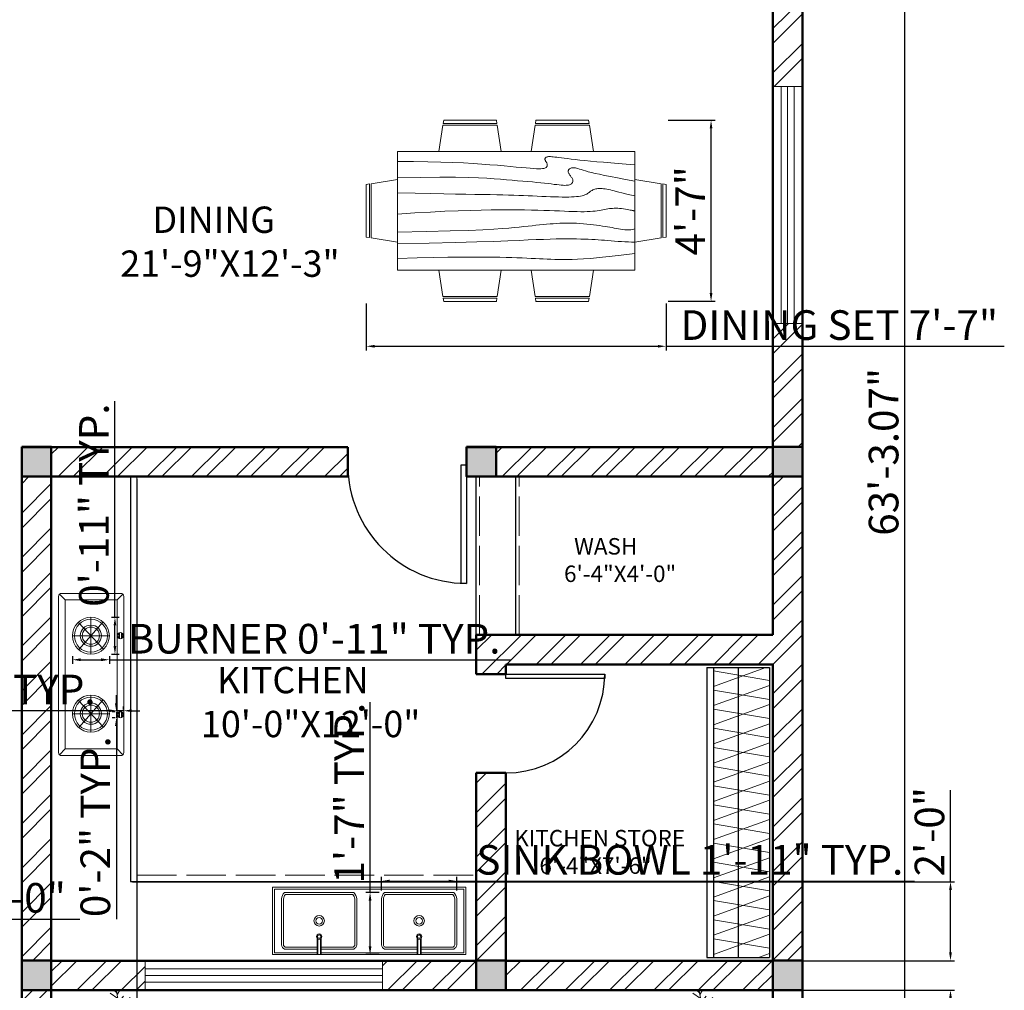
# Model space of a CAD drawing. Units: inches. Extents: x 381 to 1001, y 3003 to 3971.
# Tile 3 of 4: x 702 to 1001, y 3347 to 3641. Entities that reach past the tile are written whole.
import ezdxf

# ---------------------------------------------------------------- set-up
doc = ezdxf.new("R2010")
doc.units = ezdxf.units.IN
doc.linetypes.add('ACAD_ISO02W100', pattern=[15, 12, -3])
for name, color, linetype, lineweight in [('A-ANNO-DIMS', 2, 'Continuous', 18), ('A-AREA-IDEN', 7, 'Continuous', 18), ('A-COLS', 7, 'Continuous', 50), ('A-DOOR', 4, 'Continuous', 25), ('A-EQPM', 8, 'Continuous', 18), ('A-FLOR', 7, 'Continuous', 25), ('A-FLOR-CASE', 8, 'Continuous', 25), ('A-FLOR-CASE-HIDN', 8, 'ACAD_ISO02W100', 13), ('A-FLOR-CASE-PATT', 252, 'Continuous', 13), ('A-FLOR-FIXT', 9, 'Continuous', 18), ('A-FLOR-STRS', 7, 'Continuous', 25), ('A-FLOR-STRS-HIDN', 8, 'ACAD_ISO02W100', 13), ('A-FURN', 8, 'Continuous', 18), ('A-GLAZ', 244, 'Continuous', 18), ('A-WALL', 7, 'Continuous', 50), ('A-WALL-PATT', 252, 'Continuous', 13), ('L-PLNT', 3, 'Continuous', 13)]:
    doc.layers.add(name, color=color, linetype=linetype, lineweight=lineweight)
doc.styles.get("Standard").update_dxf_attribs({"font": 'arial.ttf'})
doc.dimstyles.new('ISO-25', dxfattribs={"dimtxt": 9, "dimasz": 2.5, "dimexe": 1.25, "dimexo": 0.625, "dimtad": 1, "dimlunit": 3, "dimtxsty": 'Standard', "dimcen": 2.5, "dimadec": 0, "dimazin": 0, "dimtfac": 1, "dimtmove": 0, "dimatfit": 3, "dimfxl": 1, "dimarcsym": 0})

# ---------------------------------------------------------------- blocks, each defined once
blk = doc.blocks.new('*U6')
for p, q in [((-40, 0), (-40, 6)), ((0, 0), (0, 6))]:
    blk.add_line(p, q)
blk.add_lwpolyline([(0, 0), (0, -40), (-1.75, -40), (-1.75, 0)], close=True)
blk.add_arc((0, 0), 40, 180, 270)
blk = doc.blocks.new('*U7')
for p, q in [((-40, 0), (-40, 6)), ((0, 0), (0, 6))]:
    blk.add_line(p, q)
blk.add_lwpolyline([(0, 0), (0, -40), (-1.75, -40), (-1.75, 0)], close=True)
blk.add_arc((0, 0), 40, 180, 270)
blk = doc.blocks.new('Dining Set - 36 x 72 in.')
for p, q in [((-22, 27.5), (-22.1562, 26.50042)), ((-22, 27.5), (-6, 27.5)), ((-5.8437, 26.49966), (-6, 27.5)), ((6, 27.5), (5.8438, 26.50042)), ((6, 27.5), (22, 27.5)), ((22.1563, 26.49966), (22, 27.5)), ((-22.2343, 26.00059), (-23.4847, 17.99762)), ((-22.2304, 26), (-5.7608, 26)), ((-5.8416, 26.5), (-22.1534, 26.5)), ((-4.5152, 17.99762), (-5.7655, 25.99926)), ((5.7657, 26.00059), (4.5153, 17.99762)), ((5.7696, 26), (22.2392, 26)), ((22.1584, 26.5), (5.8466, 26.5)), ((23.4848, 17.99762), (22.2345, 25.99926)), ((36, 18), (-36, 18)), ((-36, 18), (-36, -18)), ((36, -18), (36, 18)), ((-44.0006, 8.23428), (-35.9976, 9.48474)), ((44.0006, 8.23428), (35.9976, 9.48474)), ((-45.5, 8), (-44.5004, 8.15617)), ((-45.5, 8), (-45.5, -8)), ((-44.5, -8.15843), (-44.5, 8.15338)), ((-44, 8.23041), (-44, -8.23915)), ((44, 8.23041), (44, -8.23915)), ((44.5, -8.15843), (44.5, 8.15338)), ((45.5, 8), (44.5005, 8.15617)), ((45.5, 8), (45.5, -8)), ((-44.4997, -8.15631), (-45.5, -8)), ((-35.9976, -9.48476), (-43.9993, -8.2345)), ((35.9976, -9.48476), (43.9993, -8.2345)), ((44.4997, -8.15631), (45.5, -8)), ((-36, -18), (36, -18)), ((-22.2343, -26.0006), (-23.4847, -17.99762)), ((-4.5152, -17.99762), (-5.7655, -25.99928)), ((5.7657, -26.0006), (4.5153, -17.99762)), ((23.4848, -17.99762), (22.2345, -25.99928)), ((-22.2304, -26), (-5.7608, -26)), ((-22, -27.5), (-22.1562, -26.50044)), ((-5.8416, -26.5), (-22.1534, -26.5)), ((-5.8437, -26.49967), (-6, -27.5)), ((5.7696, -26), (22.2392, -26)), ((6, -27.5), (5.8438, -26.50044)), ((22.1584, -26.5), (5.8466, -26.5)), ((22.1563, -26.49967), (22, -27.5)), ((-22, -27.5), (-6, -27.5)), ((6, -27.5), (22, -27.5))]:
    blk.add_line(p, q)
for points in [[(-36, 15), (-31.1772, 14.97754), (-26.8079, 14.91406), (-22.8538, 14.81543), (-19.276, 14.6875), (-16.0362, 14.53613), (-13.0957, 14.36718), (-10.4159, 14.18652), (-7.9583, 14), (-5.6904, 13.81315), (-3.6035, 13.63021), (-1.6954, 13.45508), (0.0365, 13.29166), (1.5945, 13.14388), (2.9811, 13.01562), (4.1988, 12.9108), (5.25, 12.83333), (6.1393, 12.78613), (6.8802, 12.76823), (7.4883, 12.77767), (7.9792, 12.8125), (8.3685, 12.87077), (8.6719, 12.95052), (8.9049, 13.0498), (9.0833, 13.16666), (9.2205, 13.29899), (9.3216, 13.44401), (9.3895, 13.59879), (9.4271, 13.76041), (9.4373, 13.92594), (9.4232, 14.09245), (9.3875, 14.257), (9.3333, 14.41666), (9.2638, 14.56917), (9.1836, 14.71484), (9.0975, 14.85465), (9.0104, 14.98958), (8.9272, 15.1206), (8.8529, 15.2487), (8.7922, 15.37483), (8.75, 15.5), (8.7305, 15.62467), (8.7344, 15.74739), (8.7617, 15.86621), (8.8125, 15.97916), (8.8867, 16.08431), (8.9844, 16.17968), (9.1055, 16.26334), (9.25, 16.33333), (9.4189, 16.38802), (9.6172, 16.42708), (9.8506, 16.45052), (10.125, 16.45833), (10.4463, 16.45052), (10.8203, 16.42708), (11.2529, 16.38802), (11.75, 16.33333), (12.3184, 16.26318), (12.9694, 16.17838), (13.7151, 16.07991), (14.5677, 15.96875), (15.5395, 15.84586), (16.6426, 15.71224), (17.8893, 15.56884), (19.2917, 15.41666), (20.859, 15.25667), (22.5879, 15.08984), (24.4721, 14.91715), (26.5052, 14.73958), (28.6809, 14.5581), (30.9929, 14.3737), (33.4347, 14.18733), (36, 14)], [(-36, 10), (-28.9766, 10.14274), (-23.1725, 10.20442), (-18.4241, 10.19775), (-14.5677, 10.13541), (-11.4399, 10.03011), (-8.877, 9.89453), (-6.7154, 9.74137), (-4.7917, 9.58333), (-2.9698, 9.43082), (-1.2246, 9.28515), (0.4415, 9.14534), (2.026, 9.01041), (3.5266, 8.87939), (4.9408, 8.7513), (6.266, 8.62516), (7.5, 8.5), (8.6411, 8.37549), (9.6914, 8.2539), (10.6538, 8.13818), (11.5312, 8.03125), (12.3267, 7.93603), (13.043, 7.85547), (13.6831, 7.79248), (14.25, 7.75), (14.7471, 7.7303), (15.1797, 7.73307), (15.5537, 7.75732), (15.875, 7.80208), (16.1494, 7.86637), (16.3828, 7.94922), (16.5811, 8.04964), (16.75, 8.16666), (16.8944, 8.29915), (17.0143, 8.44531), (17.1089, 8.60319), (17.1771, 8.77083), (17.218, 8.94629), (17.2305, 9.1276), (17.2137, 9.31282), (17.1667, 9.5), (17.0895, 9.6875), (16.987, 9.875), (16.8649, 10.0625), (16.7292, 10.25), (16.5856, 10.4375), (16.4401, 10.625), (16.2985, 10.8125), (16.1667, 11), (16.05, 11.18733), (15.9518, 11.3737), (15.8752, 11.5581), (15.8229, 11.73958), (15.798, 11.91715), (15.8034, 12.08984), (15.842, 12.25667), (15.9167, 12.41666), (16.0295, 12.56836), (16.1784, 12.70833), (16.3605, 12.83268), (16.5729, 12.9375), (16.8127, 13.01888), (17.0768, 13.07291), (17.3625, 13.0957), (17.6667, 13.08333), (17.9894, 13.03312), (18.3418, 12.94726), (18.7382, 12.82918), (19.1927, 12.68229), (19.7195, 12.51001), (20.3327, 12.31575), (21.0465, 12.10294), (21.875, 11.875), (22.8357, 11.63354), (23.959, 11.37304), (25.2786, 11.08618), (26.8282, 10.76562), (28.6414, 10.40405), (30.752, 9.99414), (33.1936, 9.52856), (36, 9)], [(-36, 5.5), (-30.7157, 5.3348), (-26.069, 5.20963), (-21.9946, 5.11767), (-18.4271, 5.05208), (-15.3009, 5.00602), (-12.5508, 4.97265), (-10.1112, 4.94515), (-7.9167, 4.91666), (-5.909, 4.88167), (-4.0586, 4.83984), (-2.3429, 4.79215), (-0.7396, 4.73958), (0.7739, 4.6831), (2.22, 4.6237), (3.6213, 4.56233), (5, 4.5), (6.373, 4.43782), (7.7344, 4.3776), (9.0723, 4.32129), (10.375, 4.27083), (11.6309, 4.22819), (12.8281, 4.19531), (13.9551, 4.17415), (15, 4.16666), (15.954, 4.17448), (16.819, 4.19791), (17.6001, 4.23698), (18.3021, 4.29166), (18.9299, 4.36198), (19.4883, 4.44791), (19.9823, 4.54948), (20.4167, 4.66666), (20.7969, 4.79899), (21.1302, 4.94401), (21.4245, 5.09879), (21.6875, 5.26041), (21.9271, 5.42594), (22.1511, 5.59245), (22.3672, 5.757), (22.5834, 5.91666), (22.8065, 6.06868), (23.0404, 6.21093), (23.2879, 6.34147), (23.5521, 6.45833), (23.8358, 6.55957), (24.142, 6.64323), (24.4735, 6.70735), (24.8334, 6.75), (25.2235, 6.76969), (25.642, 6.76692), (26.0858, 6.74267), (26.5521, 6.69791), (27.0379, 6.63362), (27.5404, 6.55078), (28.0565, 6.45036), (28.5834, 6.33333), (29.1242, 6.19987), (29.7071, 6.04687), (30.3661, 5.87044), (31.1354, 5.66666), (32.0493, 5.43164), (33.142, 5.16146), (34.4475, 4.85221), (36, 4.5)], [(-36, -1), (-30.7915, -0.6591), (-26.0195, -0.38216), (-21.6519, -0.16284), (-17.6563, 0.00521), (-14.0005, 0.12833), (-10.6523, 0.21289), (-7.5796, 0.26522), (-4.75, 0.29166), (-2.134, 0.29793), (0.2878, 0.28711), (2.5317, 0.26163), (4.6146, 0.22396), (6.5529, 0.17651), (8.3633, 0.12174), (10.0623, 0.06209), (11.6667, 0), (13.1899, -0.06201), (14.6341, -0.1211), (15.9982, -0.17432), (17.2813, -0.21875), (18.4823, -0.25147), (19.6003, -0.26953), (20.6343, -0.27002), (21.5834, -0.25), (22.4481, -0.20768), (23.2357, -0.14584), (23.9549, -0.06836), (24.6146, 0.02083), (25.2235, 0.11784), (25.7904, 0.21875), (26.3241, 0.31966), (26.8334, 0.41666), (27.3265, 0.50618), (27.8099, 0.58593), (28.2894, 0.65397), (28.7709, 0.70833), (29.2601, 0.74707), (29.763, 0.76823), (30.2855, 0.76985), (30.8334, 0.75), (31.4088, 0.70784), (31.9994, 0.64713), (32.589, 0.57275), (33.1615, 0.48958), (33.7008, 0.4025), (34.1908, 0.3164), (34.6153, 0.23616), (34.9584, 0.16666), (35.2099, 0.11165), (35.3848, 0.07031), (35.504, 0.04069), (35.5886, 0.02083), (35.6594, 0.00879), (35.7377, 0.0026), (35.8442, 0.00032), (36, 0)], [(-36, -6.5), (-27.1843, -6.31267), (-20.084, -6.1263), (-14.469, -5.9419), (-10.1094, -5.76042), (-6.7752, -5.58285), (-4.2363, -5.41016), (-2.2629, -5.24333), (-0.625, -5.08334), (0.8708, -4.93099), (2.2715, -4.78646), (3.5872, -4.64974), (4.8281, -4.52084), (6.0046, -4.39974), (7.127, -4.28646), (8.2053, -4.18099), (9.25, -4.08334), (10.2705, -3.99382), (11.2734, -3.91407), (12.2647, -3.84603), (13.25, -3.79167), (14.2354, -3.75293), (15.2266, -3.73177), (16.2295, -3.73015), (17.25, -3.75), (18.2912, -3.79248), (19.3451, -3.85547), (20.4009, -3.93604), (21.4479, -4.03125), (22.4754, -4.13819), (23.4727, -4.25391), (24.4289, -4.37549), (25.3334, -4.5), (26.1785, -4.62492), (26.9694, -4.74935), (27.7145, -4.87281), (28.4219, -4.99479), (29.1, -5.11483), (29.7572, -5.23242), (30.4016, -5.34709), (31.0417, -5.45834), (31.6837, -5.56437), (32.3262, -5.65821), (32.9658, -5.73153), (33.599, -5.77604), (34.2224, -5.78345), (34.8327, -5.74545), (35.4264, -5.65373), (36, -5.5)], [(-36, -10), (-26.4022, -9.81299), (-18.4675, -9.62891), (-11.9839, -9.45069), (-6.7396, -9.28125), (-2.5226, -9.12354), (0.8789, -8.98047), (3.6769, -8.85498), (6.0833, -8.75), (8.2767, -8.66765), (10.3021, -8.60677), (12.1712, -8.56543), (13.8958, -8.54167), (15.4876, -8.53353), (16.9583, -8.53907), (18.3197, -8.55632), (19.5834, -8.58334), (20.7616, -8.61841), (21.8685, -8.66081), (22.9188, -8.71004), (23.9271, -8.76563), (24.9081, -8.82707), (25.8763, -8.89388), (26.8465, -8.96558), (27.8334, -9.04167), (28.8474, -9.12118), (29.8828, -9.20117), (30.93, -9.27824), (31.9792, -9.34896), (33.0205, -9.40991), (34.0443, -9.45768), (35.0407, -9.48885), (36, -9.5)], [(-36, -14.5), (-30.0881, -14.33513), (-25.0332, -14.21224), (-20.7312, -14.12647), (-17.0781, -14.07292), (-13.97, -14.04671), (-11.3027, -14.04297), (-8.9724, -14.05681), (-6.875, -14.08334), (-4.9224, -14.11833), (-3.0905, -14.16016), (-1.3709, -14.20785), (0.2448, -14.26042), (1.7647, -14.3169), (3.1973, -14.3763), (4.5507, -14.43767), (5.8333, -14.5), (7.0554, -14.5621), (8.235, -14.62175), (9.3922, -14.67652), (10.5469, -14.72396), (11.7192, -14.76164), (12.929, -14.78711), (14.1965, -14.79794), (15.5417, -14.79167), (16.9933, -14.76424), (18.6152, -14.70508), (20.4804, -14.60197), (22.6615, -14.44271), (25.2312, -14.21509), (28.2624, -13.9069), (31.8277, -13.50594), (36, -13)]]:
    blk.add_lwpolyline(points)
blk = doc.blocks.new('*U15')
for p, q in [((-10.186, 53.64), (-13.084, 55.962)), ((0, 0), (-10.5, 57)), ((-9.099, 51.782), (-6.563, 55.962)), ((-7.288, 39.707), (-21.778, 46.673)), ((-8.737, 47.138), (-17.069, 52.711)), ((-7.65, 43.423), (-2.578, 49.46)), ((-5.839, 35.992), (4.667, 48.067)), ((-5.114, 27.632), (10.463, 46.673)), ((-3.665, 19.273), (-27.574, 35.527)), ((-5.114, 28.097), (-24.676, 40.636)), ((-2.941, 16.486), (8.652, 37.85)), ((22.055, 7.198), (27.489, 32.277)), ((27, 9), (48, 36)), ((27.127, 9.056), (31.112, 35.992)), ((35.096, 32.741), (37.27, 22.524)), ((38.719, 34.134), (41.979, 28.561)), ((44.153, 36.456), (45.239, 32.741)), ((-31.5, 4.5), (-52.5, 25.5)), ((-48.585, 21.131), (-49.309, 29.026)), ((-43.513, 28.561), (-42.427, 15.558)), ((-38.442, 26.239), (-34.819, 7.663)), ((-35.544, 28.097), (-24.314, 3.947)), ((-14.533, 2.09), (-30.834, 25.31)), ((-24.314, 23.917), (-2.941, 13.7)), ((-1.129, 6.734), (9.014, 26.704)), ((3.942, 1.625), (11.187, 24.381)), ((10.101, 3.483), (17.708, 26.239)), ((16.259, 5.805), (23.142, 31.348)), ((31.836, 30.883), (32.561, 16.486)), ((40.53, 25.775), (48.862, 24.846)), ((43.791, 29.954), (51.036, 30.883)), ((-47.498, 19.737), (-55.83, 18.344)), ((-40.615, 13.7), (-55.105, 10.913)), ((-20.691, 13.7), (-1.129, 4.876)), ((29.662, 12.307), (48.137, 6.269)), ((33.285, 16.486), (48.862, 10.913)), ((36.183, 19.737), (48.137, 17.88)), ((-33.37, 6.269), (-52.207, 5.34)), ((-28.299, 3.483), (-47.86, -5.805)), ((-21.416, 3.018), (-38.079, -8.128)), ((0, 0), (-31.5, 4.5)), ((-15.982, 2.09), (-30.11, -9.521)), ((0, 0), (-22.5, -19.5)), ((-6.563, 1.161), (-21.416, -8.128)), ((0, 0), (27, 9)), ((0, 0), (18, -22.5)), ((6.478, 1.625), (26.04, -8.592)), ((11.187, 3.483), (30.749, -5.805)), ((18.07, 5.805), (35.096, -3.483)), ((24.229, 7.663), (46.688, 1.625)), ((-6.563, -5.805), (-19.967, -9.985)), ((-9.461, -8.592), (-6.201, -23.453)), ((-4.752, -3.483), (-3.665, -14.629)), ((2.493, -3.019), (-1.491, -20.202)), ((1.769, -2.555), (24.229, -9.521)), ((5.029, -6.27), (2.131, -25.775)), ((7.565, -9.056), (32.198, -14.629)), ((-17.431, -15.094), (-42.789, -18.809)), ((-22.5, -19.5), (-37.5, -45)), ((-15.257, -12.772), (-30.11, -12.772)), ((-20.691, -18.345), (-17.793, -44.352)), ((-17.069, -15.094), (-12.721, -40.172)), ((-13.446, -11.378), (-8.737, -32.741)), ((9.014, -11.378), (3.58, -35.992)), ((14.085, -16.951), (6.478, -40.172)), ((12.274, -15.094), (36.907, -18.809)), ((16.259, -19.738), (36.183, -22.989)), ((-28.299, -29.026), (-42.789, -31.348)), ((-24.314, -21.596), (-42.427, -22.06)), ((-26.849, -26.24), (-40.253, -25.775)), ((-29.023, -30.884), (-27.936, -43.887)), ((-25.038, -23.918), (-22.865, -45.281)), ((18.07, -22.524), (8.289, -45.745)), ((20.244, -30.419), (15.897, -44.816)), ((18, -22.5), (27, -52.5)), ((18.433, -22.524), (40.53, -29.026)), ((19.157, -25.311), (38.719, -33.206)), ((-30.834, -34.135), (-42.427, -35.528)), ((-34.457, -39.708), (-40.978, -42.494)), ((-32.646, -36.921), (-31.921, -44.352)), ((22.78, -37.85), (19.519, -48.532)), ((21.331, -32.741), (39.081, -40.636)), ((22.78, -38.314), (34.372, -44.816)), ((24.591, -45.745), (23.142, -50.854)), ((24.591, -43.423), (30.749, -47.603)), ((26.764, -49.925), (28.213, -50.854))]:
    blk.add_line(p, q)
blk = doc.blocks.new('*D22')
at = {"layer": 'A-ANNO-DIMS', "color": 0, "lineweight": -2, "transparency": 16777216}
for p, q in [((940.7, 3889.64), (972.35, 3889.64)), ((971.1, 3887.14), (971.1, 3133.06)), ((940.7, 3130.56), (972.35, 3130.56))]:
    blk.add_line(p, q, dxfattribs=at)
at = {"layer": 'A-ANNO-DIMS', "color": 0, "transparency": 16777216}
for points in [[(970.69, 3887.14), (971.52, 3887.14), (971.1, 3889.64)], [(970.69, 3133.06), (971.52, 3133.06), (971.1, 3130.56)]]:
    blk.add_solid(points, dxfattribs=at)
at = {"layer": 'Defpoints', "color": 0, "transparency": 16777216}
for p in [(940.08, 3889.64), (940.08, 3130.56), (971.1, 3130.56)]:
    blk.add_point(p, dxfattribs=at)
at = {"layer": 'A-ANNO-DIMS', "color": 0, "transparency": 16777216, "insert": (965.88, 3510.1), "char_height": 9, "attachment_point": 5, "rotation": 90}
blk.add_mtext('63\'-3.07"', dxfattribs=at)
blk = doc.blocks.new('WIN-72X9')
for p, q in [((72, 6.5), (0, 6.5)), ((72, 4.5), (0, 4.5)), ((72, 2.5), (0, 2.5))]:
    blk.add_line(p, q)
blk.add_lwpolyline([(72, 9), (72, 0), (0, 0), (0, 9)], close=True)
blk = doc.blocks.new('COLUMN-9X9')
h = blk.add_hatch(color=256)
h.dxf.hatch_style = 1
h.paths.add_polyline_path([(9, 9), (0, 9), (0, 0), (9, 0)])
blk.add_lwpolyline([(0, 9), (9, 9), (9, 0), (0, 0)], close=True)
blk = doc.blocks.new('SINK-BOWL-WITH-TAP')
for p, q in [((10.86, 4.95), (10.86, 0)), ((11.06, 4.79), (11.06, 0)), ((11.86, 4.79), (11.86, 0)), ((12.06, 4.95), (12.06, 0))]:
    blk.add_line(p, q)
for points in [[(12.06, 1.68), (22.01, 1.68, 0.204191), (22.91, 2.94), (22.91, 16.97, 0.131614), (22.01, 18.91), (0.9, 18.91, 0.131614), (0, 16.97), (0, 2.94, 0.204191), (0.9, 1.68), (10.86, 1.68)], [(12.06, 2.28), (21.83, 2.28, 0.163903), (22.31, 3.01), (22.31, 16.91, 0.108554), (21.72, 18.31), (1.19, 18.31, 0.108554), (0.6, 16.91), (0.6, 3.01, 0.163903), (1.09, 2.28), (10.86, 2.28)]]:
    blk.add_lwpolyline(points, format="xyb")
for centre, radius in [((11.46, 10.29), 1.59), ((11.46, 10.29), 0.993), ((11.46, 5.49), 0.805), ((11.46, 5.49), 0.505)]:
    blk.add_circle(centre, radius)
blk = doc.blocks.new('COOKTOP-BURNER')
for p, q in [((9.48, 1.55), (1.74, 9.68)), ((1.93, 1.38), (9.3, 9.85)), ((5.61, 11.23), (5.61, 0)), ((0, 5.61), (11.23, 5.61))]:
    blk.add_line(p, q)
for radius in [5.61, 5.01, 3.21, 2.61]:
    blk.add_circle((5.61, 5.61), radius)
blk = doc.blocks.new('COOKTOP-KNOB')
for p, q in [((0.64, 1.83), (0.64, 0.05)), ((1.24, 1.83), (1.24, 0.05))]:
    blk.add_line(p, q)
blk.add_circle((0.94, 0.94), 0.94)
for start, end in [(117.9584, 242.0416), (297.9584, 62.0416)]:
    blk.add_arc((0.94, 0.94), 0.64, start, end)
blk = doc.blocks.new('*D42')
at = {"layer": 'A-ANNO-DIMS', "color": 0, "lineweight": -2, "transparency": 16777216}
for p, q in [((812.27, 3376.93), (812.27, 3380.99)), ((835.18, 3376.93), (835.18, 3380.99)), ((814.77, 3379.74), (832.68, 3379.74)), ((835.18, 3379.74), (974.09, 3379.74))]:
    blk.add_line(p, q, dxfattribs=at)
at = {"layer": 'A-ANNO-DIMS', "color": 0, "transparency": 16777216}
for points in [[(814.77, 3380.16), (814.77, 3379.33), (812.27, 3379.74)], [(832.68, 3380.16), (832.68, 3379.33), (835.18, 3379.74)]]:
    blk.add_solid(points, dxfattribs=at)
at = {"layer": 'Defpoints', "color": 0, "transparency": 16777216}
for p in [(835.18, 3379.74), (812.27, 3376.31), (835.18, 3376.31)]:
    blk.add_point(p, dxfattribs=at)
at = {"layer": 'A-ANNO-DIMS', "color": 0, "transparency": 16777216, "insert": (905.89, 3385.03), "char_height": 9, "attachment_point": 5}
blk.add_mtext('SINK BOWL 1\'-11" TYP.', dxfattribs=at)
blk = doc.blocks.new('*D43')
at = {"layer": 'A-ANNO-DIMS', "color": 0, "lineweight": -2, "transparency": 16777216}
for p, q in [((808.83, 3376.31), (808.83, 3434.07)), ((811.64, 3376.31), (807.58, 3376.31)), ((808.83, 3359.9), (808.83, 3373.81)), ((811.64, 3357.4), (807.58, 3357.4))]:
    blk.add_line(p, q, dxfattribs=at)
at = {"layer": 'A-ANNO-DIMS', "color": 0, "transparency": 16777216}
for points in [[(808.41, 3373.81), (809.24, 3373.81), (808.83, 3376.31)], [(808.41, 3359.9), (809.24, 3359.9), (808.83, 3357.4)]]:
    blk.add_solid(points, dxfattribs=at)
at = {"layer": 'Defpoints', "color": 0, "transparency": 16777216}
for p in [(808.83, 3376.31), (812.27, 3376.31), (812.27, 3357.4)]:
    blk.add_point(p, dxfattribs=at)
at = {"layer": 'A-ANNO-DIMS', "color": 0, "transparency": 16777216, "insert": (803.68, 3406.44), "char_height": 9, "attachment_point": 5, "rotation": 90}
blk.add_mtext('1\'-7" TYP.', dxfattribs=at)
blk = doc.blocks.new('*D44')
at = {"layer": 'A-ANNO-DIMS', "color": 0, "lineweight": -2, "transparency": 16777216}
for p, q in [((718.48, 3448.02), (718.48, 3445.71)), ((720.98, 3446.96), (727.2, 3446.96)), ((729.7, 3448.02), (729.7, 3445.71)), ((729.7, 3446.96), (851.49, 3446.96))]:
    blk.add_line(p, q, dxfattribs=at)
at = {"layer": 'A-ANNO-DIMS', "color": 0, "transparency": 16777216}
for points in [[(720.98, 3447.38), (720.98, 3446.54), (718.48, 3446.96)], [(727.2, 3447.38), (727.2, 3446.54), (729.7, 3446.96)]]:
    blk.add_solid(points, dxfattribs=at)
at = {"layer": 'Defpoints', "color": 0, "transparency": 16777216}
for p in [(718.48, 3448.64), (729.7, 3448.64), (729.7, 3446.96)]:
    blk.add_point(p, dxfattribs=at)
at = {"layer": 'A-ANNO-DIMS', "color": 0, "transparency": 16777216, "insert": (791.85, 3452.18), "char_height": 9, "attachment_point": 5}
blk.add_mtext('BURNER 0\'-11" TYP.', dxfattribs=at)
blk = doc.blocks.new('*D45')
at = {"layer": 'A-ANNO-DIMS', "color": 0, "lineweight": -2, "transparency": 16777216}
for p, q in [((731.39, 3459.87), (731.39, 3525.47)), ((730.33, 3459.87), (732.64, 3459.87)), ((731.39, 3451.14), (731.39, 3457.37)), ((730.33, 3448.64), (732.64, 3448.64))]:
    blk.add_line(p, q, dxfattribs=at)
at = {"layer": 'A-ANNO-DIMS', "color": 0, "transparency": 16777216}
for points in [[(730.97, 3457.37), (731.8, 3457.37), (731.39, 3459.87)], [(730.97, 3451.14), (731.8, 3451.14), (731.39, 3448.64)]]:
    blk.add_solid(points, dxfattribs=at)
at = {"layer": 'Defpoints', "color": 0, "transparency": 16777216}
for p in [(729.7, 3459.87), (731.39, 3459.87), (729.7, 3448.64)]:
    blk.add_point(p, dxfattribs=at)
at = {"layer": 'A-ANNO-DIMS', "color": 0, "transparency": 16777216, "insert": (726.17, 3493.92), "char_height": 9, "attachment_point": 5, "rotation": 90}
blk.add_mtext('0\'-11" TYP.', dxfattribs=at)
blk = doc.blocks.new('*D46')
at = {"layer": 'A-ANNO-DIMS', "color": 0, "lineweight": -2, "transparency": 16777216}
for p, q in [((729.6, 3431.47), (632.26, 3431.47)), ((732.1, 3431.81), (732.1, 3432.72)), ((733.98, 3431.47), (732.1, 3431.47)), ((733.98, 3431.81), (733.98, 3432.72)), ((736.48, 3431.47), (738.98, 3431.47))]:
    blk.add_line(p, q, dxfattribs=at)
at = {"layer": 'A-ANNO-DIMS', "color": 0, "transparency": 16777216}
for points in [[(729.6, 3431.88), (729.6, 3431.05), (732.1, 3431.47)], [(736.48, 3431.88), (736.48, 3431.05), (733.98, 3431.47)]]:
    blk.add_solid(points, dxfattribs=at)
at = {"layer": 'Defpoints', "color": 0, "transparency": 16777216}
for p in [(732.1, 3431.47), (732.1, 3431.18), (733.98, 3431.18)]:
    blk.add_point(p, dxfattribs=at)
at = {"layer": 'A-ANNO-DIMS', "color": 0, "transparency": 16777216, "insert": (679.68, 3436.75), "char_height": 9, "attachment_point": 5}
blk.add_mtext('KNOB 0\'-2" TYP.', dxfattribs=at)
blk = doc.blocks.new('*D47')
at = {"layer": 'A-ANNO-DIMS', "color": 0, "lineweight": -2, "transparency": 16777216}
for p, q in [((731.82, 3433.68), (731.82, 3436.18)), ((731.47, 3431.18), (730.57, 3431.18)), ((731.82, 3431.18), (731.82, 3429.3)), ((731.47, 3429.3), (730.57, 3429.3)), ((731.82, 3426.8), (731.82, 3368.19))]:
    blk.add_line(p, q, dxfattribs=at)
at = {"layer": 'A-ANNO-DIMS', "color": 0, "transparency": 16777216}
for points in [[(731.4, 3433.68), (732.23, 3433.68), (731.82, 3431.18)], [(731.4, 3426.8), (732.23, 3426.8), (731.82, 3429.3)]]:
    blk.add_solid(points, dxfattribs=at)
at = {"layer": 'Defpoints', "color": 0, "transparency": 16777216}
for p in [(732.1, 3431.18), (731.82, 3429.3), (732.1, 3429.3)]:
    blk.add_point(p, dxfattribs=at)
at = {"layer": 'A-ANNO-DIMS', "color": 0, "transparency": 16777216, "insert": (726.6, 3396.25), "char_height": 9, "attachment_point": 5, "rotation": 90}
blk.add_mtext('0\'-2" TYP.', dxfattribs=at)
blk = doc.blocks.new('*D48')
at = {"layer": 'A-ANNO-DIMS', "color": 0, "lineweight": -2, "transparency": 16777216}
for p, q in [((807.69, 3555.18), (807.69, 3540.91)), ((898.69, 3555.18), (898.69, 3540.91)), ((810.19, 3542.16), (896.19, 3542.16)), ((898.69, 3542.16), (1001.36, 3542.16))]:
    blk.add_line(p, q, dxfattribs=at)
at = {"layer": 'A-ANNO-DIMS', "color": 0, "transparency": 16777216}
for points in [[(810.19, 3542.57), (810.19, 3541.74), (807.69, 3542.16)], [(896.19, 3542.57), (896.19, 3541.74), (898.69, 3542.16)]]:
    blk.add_solid(points, dxfattribs=at)
at = {"layer": 'Defpoints', "color": 0, "transparency": 16777216}
for p in [(807.69, 3555.81), (898.69, 3555.81), (898.69, 3542.16)]:
    blk.add_point(p, dxfattribs=at)
at = {"layer": 'A-ANNO-DIMS', "color": 0, "transparency": 16777216, "insert": (951.27, 3547.43), "char_height": 9, "attachment_point": 5}
blk.add_mtext('DINING SET 7\'-7"', dxfattribs=at)
blk = doc.blocks.new('*D49')
at = {"layer": 'A-ANNO-DIMS', "color": 0, "lineweight": -2, "transparency": 16777216}
for p, q in [((899.31, 3610.81), (913.59, 3610.81)), ((912.34, 3558.31), (912.34, 3608.31)), ((899.31, 3555.81), (913.59, 3555.81))]:
    blk.add_line(p, q, dxfattribs=at)
at = {"layer": 'A-ANNO-DIMS', "color": 0, "transparency": 16777216}
for points in [[(911.92, 3608.31), (912.75, 3608.31), (912.34, 3610.81)], [(911.92, 3558.31), (912.75, 3558.31), (912.34, 3555.81)]]:
    blk.add_solid(points, dxfattribs=at)
at = {"layer": 'Defpoints', "color": 0, "transparency": 16777216}
for p in [(898.69, 3610.81), (912.34, 3610.81), (898.69, 3555.81)]:
    blk.add_point(p, dxfattribs=at)
at = {"layer": 'A-ANNO-DIMS', "color": 0, "transparency": 16777216, "insert": (907.21, 3583.31), "char_height": 9, "attachment_point": 5, "rotation": 90}
blk.add_mtext('4\'-7"', dxfattribs=at)
blk = doc.blocks.new('*D50')
at = {"layer": 'A-ANNO-DIMS', "color": 0, "lineweight": -2, "transparency": 16777216}
for p, q in [((535.37, 3376.58), (535.37, 3366.95)), ((595.37, 3376.58), (595.37, 3366.95)), ((537.87, 3368.2), (592.87, 3368.2)), ((595.37, 3368.2), (720.75, 3368.2))]:
    blk.add_line(p, q, dxfattribs=at)
at = {"layer": 'A-ANNO-DIMS', "color": 0, "transparency": 16777216}
for points in [[(537.87, 3368.62), (537.87, 3367.79), (535.37, 3368.2)], [(592.87, 3368.62), (592.87, 3367.79), (595.37, 3368.2)]]:
    blk.add_solid(points, dxfattribs=at)
at = {"layer": 'Defpoints', "color": 0, "transparency": 16777216}
for p in [(535.37, 3377.2), (595.37, 3377.2), (595.37, 3368.2)]:
    blk.add_point(p, dxfattribs=at)
at = {"layer": 'A-ANNO-DIMS', "color": 0, "transparency": 16777216, "insert": (659.31, 3373.48), "char_height": 9, "attachment_point": 5}
blk.add_mtext('COFFEE TABLE 5\'-0"', dxfattribs=at)
blk = doc.blocks.new('*D57')
at = {"layer": 'A-ANNO-DIMS', "color": 0, "lineweight": -2, "transparency": 16777216}
for p, q in [((703.7, 3346.64), (986.28, 3346.64)), ((985.03, 3298.06), (985.03, 3344.14)), ((703.7, 3295.56), (986.28, 3295.56))]:
    blk.add_line(p, q, dxfattribs=at)
at = {"layer": 'A-ANNO-DIMS', "color": 0, "transparency": 16777216}
for points in [[(984.61, 3344.14), (985.44, 3344.14), (985.03, 3346.64)], [(984.61, 3298.06), (985.44, 3298.06), (985.03, 3295.56)]]:
    blk.add_solid(points, dxfattribs=at)
at = {"layer": 'Defpoints', "color": 0, "transparency": 16777216}
for p in [(703.08, 3346.64), (985.03, 3346.64), (703.08, 3295.56)]:
    blk.add_point(p, dxfattribs=at)
at = {"layer": 'A-ANNO-DIMS', "color": 0, "transparency": 16777216, "insert": (979.81, 3321.1), "char_height": 9, "attachment_point": 5, "rotation": 90}
blk.add_mtext('4\'-3"', dxfattribs=at)
blk = doc.blocks.new('*D59')
at = {"layer": 'A-ANNO-DIMS', "color": 0, "lineweight": -2, "transparency": 16777216}
for p, q in [((712.08, 3502.01), (712.08, 3002.98)), ((738.08, 3501.94), (738.08, 3002.98)), ((714.58, 3004.23), (735.58, 3004.23))]:
    blk.add_line(p, q, dxfattribs=at)
at = {"layer": 'A-ANNO-DIMS', "color": 0, "transparency": 16777216}
for points in [[(714.58, 3004.64), (714.58, 3003.81), (712.08, 3004.23)], [(735.58, 3004.64), (735.58, 3003.81), (738.08, 3004.23)]]:
    blk.add_solid(points, dxfattribs=at)
at = {"layer": 'Defpoints', "color": 0, "transparency": 16777216}
for p in [(712.08, 3502.64), (738.08, 3502.56), (738.08, 3004.23)]:
    blk.add_point(p, dxfattribs=at)
at = {"layer": 'A-ANNO-DIMS', "color": 0, "transparency": 16777216, "insert": (725.08, 3009.37), "char_height": 9, "attachment_point": 5}
blk.add_mtext('2\'-2"', dxfattribs=at)
blk = doc.blocks.new('*D60')
at = {"layer": 'A-ANNO-DIMS', "color": 0, "lineweight": -2, "transparency": 16777216}
for p, q in [((985.03, 3379.56), (985.03, 3407.39)), ((736.7, 3379.56), (986.28, 3379.56)), ((985.03, 3358.06), (985.03, 3377.06)), ((712.7, 3355.56), (986.28, 3355.56))]:
    blk.add_line(p, q, dxfattribs=at)
at = {"layer": 'A-ANNO-DIMS', "color": 0, "transparency": 16777216}
for points in [[(984.61, 3377.06), (985.44, 3377.06), (985.03, 3379.56)], [(984.61, 3358.06), (985.44, 3358.06), (985.03, 3355.56)]]:
    blk.add_solid(points, dxfattribs=at)
at = {"layer": 'Defpoints', "color": 0, "transparency": 16777216}
for p in [(736.08, 3379.56), (985.03, 3379.56), (712.08, 3355.56)]:
    blk.add_point(p, dxfattribs=at)
at = {"layer": 'A-ANNO-DIMS', "color": 0, "transparency": 16777216, "insert": (979.81, 3394.73), "char_height": 9, "attachment_point": 5, "rotation": 90}
blk.add_mtext('2\'-0"', dxfattribs=at)

msp = doc.modelspace()

# ---------------------------------------------------------------- hatches: boundary and pattern name
at = {"layer": 'A-FLOR-CASE-PATT'}
h = msp.add_hatch(dxfattribs=at)
h.set_pattern_fill('ANSI31', color=256, scale=1.72204, angle=-25.1679, style=0)
h.paths.add_polyline_path([(913.078, 3356.565), (930.078, 3356.565), (930.078, 3444.565), (913.078, 3444.565)])
h = msp.add_hatch(dxfattribs=at)
h.set_pattern_fill('ANSI31', color=256, scale=1.80506, angle=125.416, style=0)
h.paths.add_polyline_path([(913.078, 3356.565), (930.078, 3356.565), (930.078, 3444.565), (913.078, 3444.565)])
at = {"layer": 'A-WALL-PATT'}
h = msp.add_hatch(dxfattribs=at)
h.set_pattern_fill('ANSI32', color=256)
h.paths.add_polyline_path([(652.078, 3667.565), (487.078, 3667.565), (487.078, 3658.565), (631.078, 3658.565), (631.078, 3655.565), (634.678, 3655.565), (640.078, 3655.565), (640.078, 3658.565), (652.078, 3658.565)])
h.paths.add_polyline_path([(487.078, 3658.637), (478.078, 3658.637), (478.078, 3634.565), (487.078, 3634.565)])
h.paths.add_polyline_path([(487.078, 3703.565), (478.078, 3703.565), (478.078, 3667.637), (487.078, 3667.637)])
h.paths.add_polyline_path([(661.078, 3811.637), (652.078, 3811.637), (652.078, 3706.565), (661.078, 3706.565)])
h.paths.add_polyline_path([(661.078, 3670.565), (655.678, 3670.565), (652.078, 3670.565), (652.078, 3667.637), (661.078, 3667.637)])
h.paths.add_polyline_path([(487.078, 3811.637), (478.078, 3811.637), (478.078, 3775.565), (487.078, 3775.565)])
h.paths.add_polyline_path([(487.078, 3880.565), (478.078, 3880.565), (478.078, 3820.637), (487.078, 3820.637)])
h.paths.add_polyline_path([(661.078, 3880.637), (652.078, 3880.637), (652.078, 3820.637), (661.078, 3820.637)])
h.paths.add_polyline_path([(652.078, 3820.565), (568.078, 3820.565), (568.078, 3823.565), (563.578, 3823.565), (562.078, 3823.565), (562.078, 3820.565), (559.078, 3820.565), (559.078, 3811.565), (652.078, 3811.565), (652.078, 3811.637)])
h.paths.add_polyline_path([(523.078, 3820.565), (487.078, 3820.565), (487.078, 3811.565), (523.078, 3811.565)])
h.paths.add_polyline_path([(619.798, 3889.565), (487.078, 3889.565), (487.078, 3880.565), (562.078, 3880.565), (562.078, 3853.565), (568.078, 3853.565), (568.078, 3880.565), (619.798, 3880.565)])
h.paths.add_polyline_path([(652.078, 3889.565), (640.798, 3889.565), (640.798, 3880.565), (652.078, 3880.565), (652.078, 3880.637)])
h.paths.add_polyline_path([(757.078, 3889.565), (661.078, 3889.565), (661.078, 3880.565), (757.078, 3880.565)])
h.paths.add_polyline_path([(766.078, 3880.637), (757.078, 3880.637), (757.078, 3820.637), (766.078, 3820.637)])
h.paths.add_polyline_path([(773.578, 3889.565), (766.078, 3889.565), (766.078, 3880.565), (773.578, 3880.565)])
h.paths.add_polyline_path([(931.078, 3889.565), (794.578, 3889.565), (794.578, 3880.565), (850.078, 3880.565), (850.078, 3853.565), (856.078, 3853.565), (856.078, 3880.565), (931.078, 3880.565)])
h.paths.add_polyline_path([(859.078, 3820.565), (856.078, 3820.565), (856.078, 3823.565), (850.078, 3823.565), (850.078, 3820.565), (766.078, 3820.565), (766.078, 3811.565), (859.078, 3811.565)])
h.paths.add_polyline_path([(940.078, 3880.637), (931.078, 3880.637), (931.078, 3820.637), (940.078, 3820.637)])
h.paths.add_polyline_path([(931.078, 3820.565), (895.078, 3820.565), (895.078, 3811.565), (931.078, 3811.565)])
h.paths.add_polyline_path([(940.078, 3811.637), (931.078, 3811.637), (931.078, 3775.565), (940.078, 3775.565)])
h.paths.add_polyline_path([(766.078, 3811.637), (757.078, 3811.637), (757.078, 3706.565), (766.078, 3706.565)])
h.paths.add_polyline_path([(940.078, 3703.565), (931.078, 3703.565), (931.078, 3667.637), (940.078, 3667.637)])
h.paths.add_polyline_path([(931.078, 3667.565), (766.078, 3667.565), (766.078, 3658.565), (931.078, 3658.565)])
h.paths.add_polyline_path([(940.078, 3658.637), (931.078, 3658.637), (931.078, 3621.065), (940.078, 3621.065)])
h.paths.add_polyline_path([(940.078, 3549.065), (931.078, 3549.065), (931.078, 3511.637), (940.078, 3511.637)])
h.paths.add_polyline_path([(931.078, 3511.565), (847.078, 3511.565), (847.078, 3502.565), (931.078, 3502.565)])
h.paths.add_polyline_path([(802.078, 3511.565), (712.078, 3511.565), (712.078, 3502.565), (802.078, 3502.565)])
h.paths.add_polyline_path([(712.078, 3502.637), (703.078, 3502.637), (703.078, 3355.637), (712.078, 3355.637)])
h.paths.add_polyline_path([(740.578, 3355.565), (712.078, 3355.565), (712.078, 3346.565), (740.578, 3346.565)])
h.paths.add_polyline_path([(841.078, 3355.565), (812.578, 3355.565), (812.578, 3346.565), (841.078, 3346.565)])
h.paths.add_polyline_path([(850.078, 3412.565), (841.078, 3412.565), (841.078, 3355.637), (850.078, 3355.637)], flags=17)
h.paths.add_polyline_path([(940.078, 3502.637), (931.078, 3502.637), (931.078, 3454.565), (841.078, 3454.565), (841.078, 3442.565), (850.078, 3442.565), (850.078, 3445.565), (931.078, 3445.565), (931.078, 3355.637), (940.078, 3355.637)])
h.paths.add_polyline_path([(931.078, 3355.565), (850.078, 3355.565), (850.078, 3346.565), (931.078, 3346.565)])
h.paths.add_polyline_path([(712.078, 3346.637), (703.078, 3346.637), (703.078, 3304.565), (700.078, 3304.565), (700.078, 3295.565), (712.078, 3295.565)])
h.paths.add_polyline_path([(622.078, 3202.565), (487.078, 3202.565), (487.078, 3193.565), (622.078, 3193.565)])
h.paths.add_polyline_path([(487.078, 3295.637), (478.078, 3295.637), (478.078, 3202.637), (487.078, 3202.637)])
h.paths.add_polyline_path([(712.078, 3295.565), (703.078, 3295.565), (703.078, 3202.565), (712.078, 3202.565)])

# ---------------------------------------------------------------- linework, layer by layer
at = {"layer": 'A-EQPM'}
for p, q in [((716.291, 3465.114), (714.554, 3466.851)), ((732.047, 3465.114), (733.783, 3466.851)), ((716.291, 3419.861), (714.554, 3418.125)), ((732.047, 3419.861), (733.783, 3418.125))]:
    msp.add_line(p, q, dxfattribs=at)
msp.add_lwpolyline([(714.291, 3466.214, -0.4142136), (715.191, 3467.114), (733.147, 3467.114, -0.4142136), (734.047, 3466.214), (734.047, 3418.761, -0.4142136), (733.147, 3417.861), (715.191, 3417.861, -0.4142136), (714.291, 3418.761)], format="xyb", close=True, dxfattribs=at)
msp.add_lwpolyline([(716.291, 3465.114), (732.047, 3465.114), (732.047, 3419.861), (716.291, 3419.861)], close=True, dxfattribs=at)
at = {"layer": 'A-FLOR'}
for p, q in [((931.078, 3346.565), (940.078, 3199.565)), ((931.078, 3199.565), (940.078, 3346.565))]:
    msp.add_line(p, q, dxfattribs=at)
at = {"layer": 'A-FLOR-CASE'}
for p, q in [((736.078, 3502.565), (736.078, 3379.565)), ((911.078, 3444.565), (930.078, 3444.565)), ((911.078, 3444.565), (911.078, 3356.565)), ((913.078, 3444.565), (913.078, 3356.565)), ((920.578, 3444.565), (920.578, 3356.565)), ((930.078, 3444.565), (930.078, 3356.565)), ((736.078, 3379.565), (841.078, 3379.565)), ((911.078, 3356.565), (930.078, 3356.565))]:
    msp.add_line(p, q, dxfattribs=at)
at = {"layer": 'A-FLOR-CASE-HIDN'}
for p, q in [((738.078, 3502.565), (738.078, 3381.565)), ((738.078, 3381.565), (841.078, 3381.565))]:
    msp.add_line(p, q, dxfattribs=at)
at = {"layer": 'A-FLOR-FIXT'}
msp.add_lwpolyline([(779.199, 3377.902), (837.901, 3377.902), (837.901, 3357.397), (779.199, 3357.397)], close=True, dxfattribs=at)
for points in [[(792.778, 3357.997), (779.799, 3357.997), (779.799, 3377.302), (837.301, 3377.302), (837.301, 3357.997), (824.322, 3357.997)], [(823.122, 3357.997), (793.978, 3357.997)]]:
    msp.add_lwpolyline(points, dxfattribs=at)
at = {"layer": 'A-FLOR-STRS'}
for p, q in [((841.078, 3454.565), (841.078, 3502.565)), ((853.078, 3454.565), (853.078, 3502.565))]:
    msp.add_line(p, q, dxfattribs=at)
at = {"layer": 'A-FLOR-STRS-HIDN'}
for p, q in [((842.078, 3454.565), (842.078, 3502.565)), ((854.078, 3454.565), (854.078, 3502.565))]:
    msp.add_line(p, q, dxfattribs=at)
at = {"layer": 'A-WALL'}
for p, q in [((940.078, 3889.565), (940.078, 3130.565)), ((931.078, 3658.565), (931.078, 3511.565)), ((703.078, 3511.565), (802.078, 3511.565)), ((703.078, 3511.565), (703.078, 3304.565)), ((802.078, 3502.565), (802.078, 3511.565)), ((838.078, 3502.565), (838.078, 3511.565)), ((838.078, 3511.565), (931.078, 3511.565)), ((712.078, 3502.565), (802.078, 3502.565)), ((712.078, 3502.565), (712.078, 3355.565)), ((838.078, 3502.565), (841.078, 3502.565)), ((841.078, 3502.565), (931.078, 3502.565)), ((931.078, 3502.565), (931.078, 3454.565)), ((841.078, 3454.565), (841.078, 3442.565)), ((841.078, 3454.565), (931.078, 3454.565)), ((850.078, 3445.565), (931.078, 3445.565)), ((850.078, 3445.565), (850.078, 3442.565)), ((931.078, 3445.565), (931.078, 3355.565)), ((850.078, 3442.565), (841.078, 3442.565)), ((850.078, 3412.565), (841.078, 3412.565)), ((841.078, 3412.565), (841.078, 3355.565)), ((850.078, 3412.565), (850.078, 3355.565)), ((712.078, 3355.565), (841.078, 3355.565)), ((850.078, 3355.565), (931.078, 3355.565)), ((712.078, 3346.565), (940.078, 3346.565)), ((712.078, 3346.565), (712.078, 3184.565)), ((931.078, 3346.565), (931.078, 3193.565))]:
    msp.add_line(p, q, dxfattribs=at)

# ---------------------------------------------------------------- block references
at = {"layer": 'A-COLS'}
for p in [(703.078, 3502.637), (838.078, 3502.637), (931.078, 3502.637), (703.078, 3346.637), (841.078, 3346.637), (931.078, 3346.637)]:
    msp.add_blockref('COLUMN-9X9', p, dxfattribs=at)
at = {"layer": 'A-DOOR', "xscale": 0.9, "yscale": 0.9, "zscale": 0.9}
msp.add_blockref('*U7', (838.078, 3506.165), dxfattribs=at)
at = {"layer": 'A-DOOR', "xscale": 0.75, "yscale": 0.75, "zscale": 0.75, "rotation": 90}
msp.add_blockref('*U6', (850.078, 3442.565), dxfattribs=at)
at = {"layer": 'A-EQPM'}
for name, p in [('COOKTOP-BURNER', (718.476, 3448.643)), ('COOKTOP-KNOB', (732.098, 3453.316)), ('COOKTOP-BURNER', (718.476, 3424.973))]:
    msp.add_blockref(name, p, dxfattribs=at)
at = {"layer": 'A-EQPM', "rotation": 180}
msp.add_blockref('COOKTOP-KNOB', (733.977, 3431.184), dxfattribs=at)
at = {"layer": 'A-FLOR-FIXT'}
for p in [(781.921, 3357.397), (812.265, 3357.397)]:
    msp.add_blockref('SINK-BOWL-WITH-TAP', p, dxfattribs=at)
at = {"layer": 'A-FURN'}
msp.add_blockref('Dining Set - 36 x 72 in.', (853.187, 3583.306), dxfattribs=at)
at = {"layer": 'A-GLAZ', "rotation": 89.99999999999996}
msp.add_blockref('WIN-72X9', (940.078, 3549.065), dxfattribs=at)
at = {"layer": 'A-GLAZ'}
msp.add_blockref('WIN-72X9', (740.578, 3346.565), dxfattribs=at)
at = {"layer": 'L-PLNT', "xscale": 0.2802404577001134, "yscale": 0.2802404577001134, "zscale": 0.2802404577001134}
for p in [(734.683, 3330.914), (911.589, 3330.914)]:
    msp.add_blockref('*U15', p, dxfattribs=at)

# ---------------------------------------------------------------- texts
at = {"layer": 'A-AREA-IDEN', "attachment_point": 1}
for s, width, insert, char_height in [('    DINING\\P21\'-9"X12\'-3"', 69.00419, (732.994, 3584.587), 8), ('  WASH\\P6\'-4"X4\'-0"', 31.66639, (867.715, 3483.905), 5), ('  KITCHEN\\P10\'-0"X12\'-0"', 63.36363, (757.499, 3444.78), 8), ('KITCHEN STORE\\P     6\'-4"X7\'-6"', 56.82697, (852.605, 3395.272), 5)]:
    msp.add_mtext_dynamic_manual_height_columns(s, width=width, gutter_width=12.5, heights=[0], dxfattribs=dict(at, insert=insert, char_height=char_height))

# ---------------------------------------------------------------- dimensions: what is measured, and where the dimension line sits
at = {"layer": 'A-ANNO-DIMS'}
for base, p1, p2, override, picture, middle in [((971.102, 3130.565), (940.078, 3889.637), (940.078, 3130.565), {"dimclrd": 0, "dimclre": 0, "dimclrt": 0}, '*D22', (965.879, 3510.101)), ((912.337, 3610.806), (898.687, 3555.806), (898.687, 3610.806), {"dimdec": 1, "dimlfac": 1, "dimrnd": 0, "dimzin": 1, "dimdsep": 46, "dimlunit": 4, "dimfrac": 2}, '*D49', (907.212, 3583.306)), ((985.028, 3379.565), (712.078, 3355.565), (736.078, 3379.565), {"dimdec": 1, "dimlfac": 1, "dimrnd": 0, "dimzin": 1, "dimdsep": 46, "dimlunit": 4, "dimfrac": 2}, '*D60', (979.808, 3394.729)), ((985.028, 3346.637), (703.078, 3295.565), (703.078, 3346.637), {"dimdec": 1, "dimlfac": 1, "dimrnd": 0, "dimzin": 1, "dimdsep": 46, "dimlunit": 4, "dimfrac": 2}, '*D57', (979.805, 3321.101))]:
    dim = msp.add_linear_dim(base=base, p1=p1, p2=p2, angle=90, dimstyle='ISO-25', override=override, dxfattribs=at)
    dim.commit()
    dim.dimension.update_dxf_attribs({"geometry": picture, "text_midpoint": middle})
for base, p1, p2, text, picture, middle in [((898.687, 3542.156), (807.687, 3555.806), (898.687, 3555.806), 'DINING SET <>', '*D48', (951.272, 3547.435)), ((729.703, 3446.959), (718.476, 3448.643), (729.703, 3448.643), 'BURNER <> TYP.', '*D44', (791.847, 3452.179)), ((835.178, 3379.745), (812.265, 3376.308), (835.178, 3376.308), 'SINK BOWL <> TYP.', '*D42', (905.886, 3385.026)), ((595.37, 3368.202), (535.37, 3377.202), (595.37, 3377.202), 'COFFEE TABLE <>', '*D50', (659.309, 3373.483))]:
    dim = msp.add_linear_dim(base=base, p1=p1, p2=p2, text=text, dimstyle='ISO-25', override={"dimdec": 1, "dimlfac": 1, "dimrnd": 0, "dimzin": 1, "dimdsep": 46, "dimlunit": 4, "dimfrac": 2}, dxfattribs=at)
    dim.commit()
    dim.dimension.update_dxf_attribs({"geometry": picture, "text_midpoint": middle})
for base, p1, p2, angle, text, picture, middle in [((731.387, 3459.87), (729.703, 3448.643), (729.703, 3459.87), 90, '<> TYP.', '*D45', (726.167, 3493.921)), ((732.098, 3431.466), (733.977, 3431.184), (732.098, 3431.184), 180, 'KNOB <> TYP.', '*D46', (679.68, 3436.748)), ((731.816, 3429.304), (732.098, 3431.184), (732.098, 3429.304), 270, '<> TYP.', '*D47', (726.595, 3396.25)), ((808.828, 3376.308), (812.265, 3357.397), (812.265, 3376.308), 90, '<> TYP.', '*D43', (803.682, 3406.439))]:
    dim = msp.add_linear_dim(base=base, p1=p1, p2=p2, angle=angle, text=text, dimstyle='ISO-25', override={"dimdec": 1, "dimlfac": 1, "dimrnd": 0, "dimzin": 1, "dimdsep": 46, "dimlunit": 4, "dimfrac": 2}, dxfattribs=at)
    dim.commit()
    dim.dimension.update_dxf_attribs({"geometry": picture, "text_midpoint": middle})
dim = msp.add_linear_dim(base=(738.078, 3004.226), p1=(712.078, 3502.637), p2=(738.078, 3502.565), dimstyle='ISO-25', override={"dimdec": 1, "dimlfac": 1, "dimrnd": 0, "dimzin": 1, "dimdsep": 46, "dimlunit": 4, "dimfrac": 2}, dxfattribs=at)
dim.commit()
dim.dimension.update_dxf_attribs({"geometry": '*D59', "text_midpoint": (725.078, 3009.37)})

doc.saveas('drawing.dxf')
